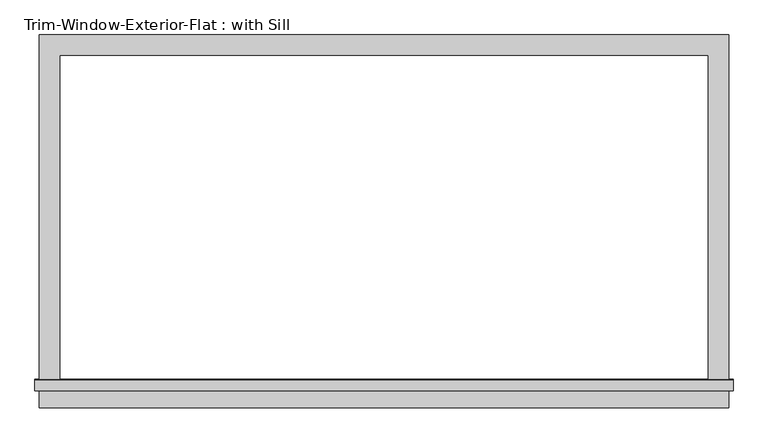
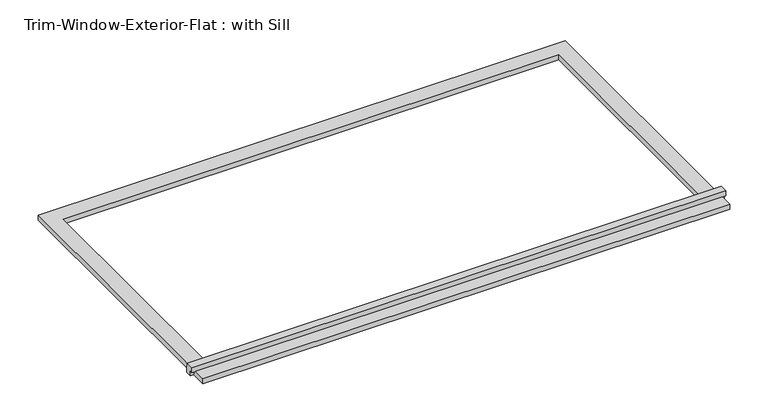
"""IFC4 building model written with IfcOpenShell, lengths in millimetres: proxy geometry, Trim-Window-Exterior-Flat : with Sill."""

from ifc_helpers import new_model, si_unit, frame, origin, origin_with_axes, place, context, project, spatial, polyline, outline, extrude, source, transform, mapped, element, save


def trim_window_exterior_flat_with_sill_3c945769(model_context):
    return source(origin(), model_context, "Body", "SweptSolid", [
        extrude(outline(polyline([(971.55, -936.5823709), (971.55, -993.7323709), (-971.55, -993.7323709), (-971.55, -936.5823709), (971.55, -936.5823709)])), origin_with_axes(), (0.0, 0.0, 1.0), 19.05),
        extrude(outline(polyline([(-946.15, 38.1), (-916.8580645, 38.1), (-914.4, 19.05), (-914.4, 0.0), (-936.5823709, 0.0), (-936.5823709, 19.05), (-946.15, 19.05), (-946.15, 38.1)])), frame((-984.25, 0.0, 0.0), z_axis=(1.0, 0.0, 0.0), x_axis=(0.0, 1.0, 0.0)), (0.0, 0.0, 1.0), 1968.5),
        extrude(outline(polyline([(-971.55, 57.15), (971.55, 57.15), (971.55, -914.4), (914.4, -914.4), (914.4, 0.0), (-914.4, 0.0), (-914.4, -914.4), (-971.55, -914.4), (-971.55, 57.15)])), origin_with_axes(), (0.0, 0.0, 1.0), 19.05),
    ])


if __name__ == "__main__":
    model = new_model("IFC4")
    model_context = context("Model", 3, world=origin())
    ifc_project = project(units=[si_unit("LENGTHUNIT", "METRE", prefix="MILLI")], contexts=[model_context])
    site = spatial("IfcSite", under=ifc_project)
    building = spatial("IfcBuilding", under=site)
    placement = place(None, origin())
    trim_window_exterior_flat_with_sill_shape = trim_window_exterior_flat_with_sill_3c945769(model_context)
    element("IfcBuildingElementProxy", 1, Name="Trim-Window-Exterior-Flat : with Sill", ObjectType="Trim-Window-Exterior-Flat : with Sill", at=placement, inside=building, context=model_context, shape_type="MappedRepresentation", body=[
        mapped(trim_window_exterior_flat_with_sill_shape, transform((0.0, 0.0, 0.0), x_axis=(1.0, 0.0, 0.0), y_axis=(0.0, 1.0, 0.0), z_axis=(0.0, 0.0, 1.0))),
    ])
    save(model, "model.ifc")

# Revit data of these elements
# Type "Trim-Window-Exterior-Flat : with Sill"
#   Trim Width = 0' - 2 1/4"
#   Trim Thickness_Picture Frame = 0' - 1 1/4"
#   Trim Thickness_with Sill = 0' - 0 3/4"
#   Sill Thickness = 0' - 1 1/4"
#   Opening Width [instance default] = 2' - 0"
#   Opening Height [instance default] = 3' - 0"
#   Default Elevation = 4' - 0"
#   Sill = yes
#   Picture Frame = no
#   Trim Material [instance default] = none
# Element 1 (IfcBuildingElementProxy, "Trim-Window-Exterior-Flat : with Sill")
#   Opening Width = 6' - 0"
#   Trim Material = Clad - White
#   Materials on its faces: "Clad - White"
# Materials
#   "Clad - White": class "Wood", colour RGB 242 242 238, transparency 0, Cost = 0
